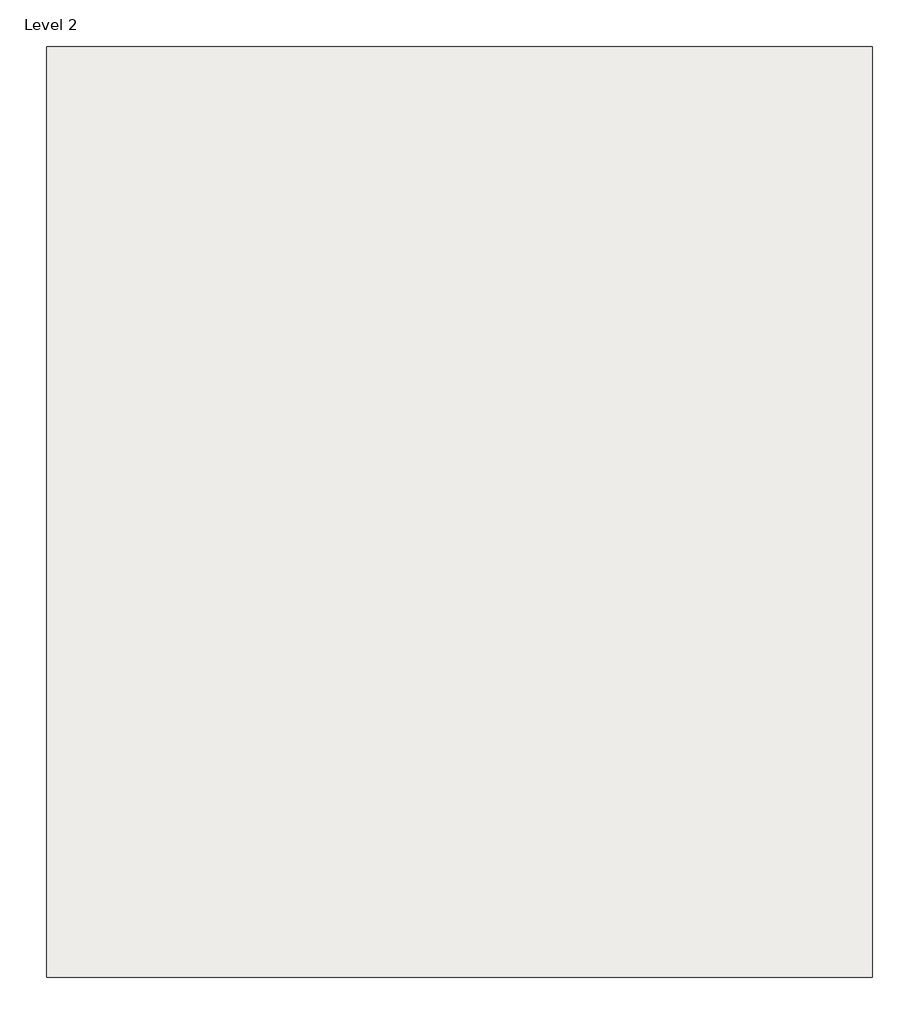
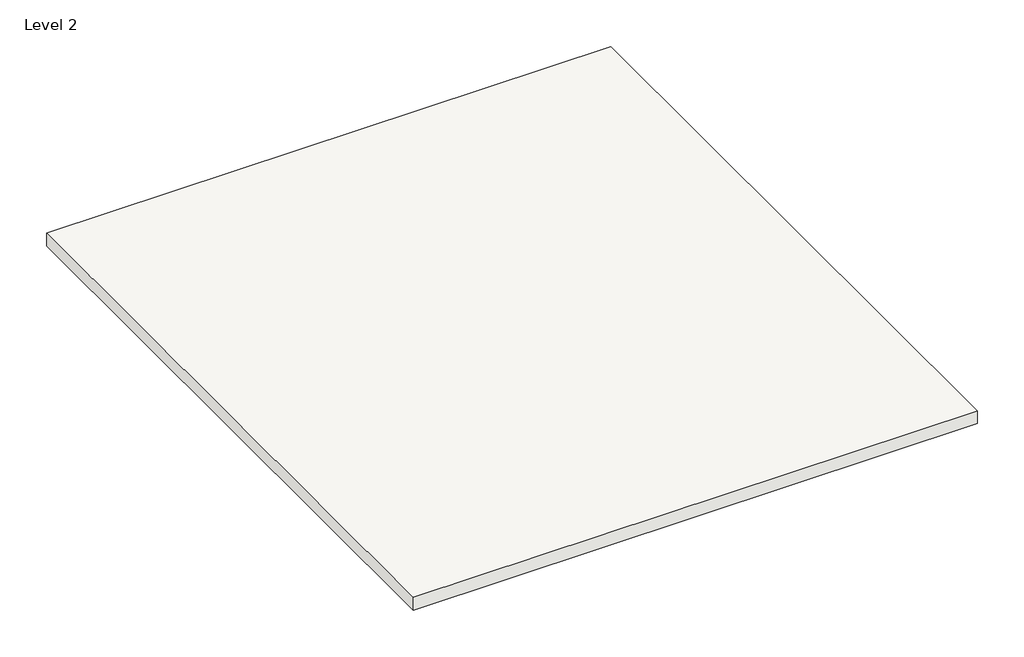
# One storey: 1 roof.
"""IFC4 building model written with IfcOpenShell, lengths in millimetres."""

from ifc_helpers import new_model, si_unit, frame, origin, place, context, project, spatial, polyline, outline, extrude, element, save

model = new_model("IFC4")

# Units and contexts
model_context = context("Model", 3, world=origin())
ifc_project = project(units=[si_unit("LENGTHUNIT", "METRE", prefix="MILLI")], contexts=[model_context])

# Site, building, storey
site = spatial("IfcSite", under=ifc_project)
building = spatial("IfcBuilding", under=site)
storey = spatial("IfcBuildingStorey", under=building, Name="Level 2", Elevation=3048.0)

# Roof
placement = place(None, origin())
element("IfcRoof", 1, ObjectType="Generic - 12\"", at=placement, inside=storey, context=model_context, shape_type="SweptSolid", body=[
    extrude(outline(polyline([(-2881.2648609, -380.8198949), (-15530.4648609, -380.8198949), (-15530.4648609, 13868.5801051), (-2881.2648609, 13868.5801051), (-2881.2648609, -380.8198949)])), frame((0.0, 0.0, 3048.0), z_axis=(0.0, 0.0, 1.0), x_axis=(1.0, 0.0, 0.0)), (0.0, 0.0, 1.0), 304.8),
])

save(model, "model.ifc")

# Revit data of these elements
# Type "Generic - 12\""
#   Assembly Code = "B1020"
#   Layers, outside or top first: 1' - 0" no material (function 1)
# Element 1 (IfcRoof, "Generic - 12\"")
#   built-in parameter 1001705 = 11 (stored number, unit not read)
#   built-in parameter 1001710 = 33615
#   Phase Created = New Construction
#   Materials on its faces: "Default Roof"
# Materials
#   "Default Roof": colour RGB 88 101 114, transparency 0
